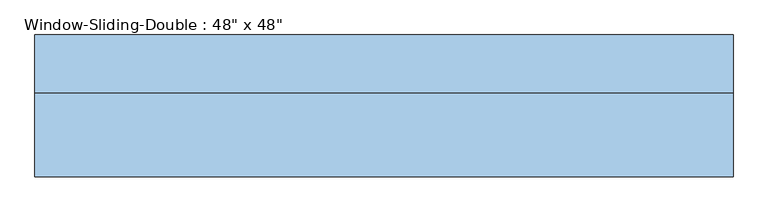
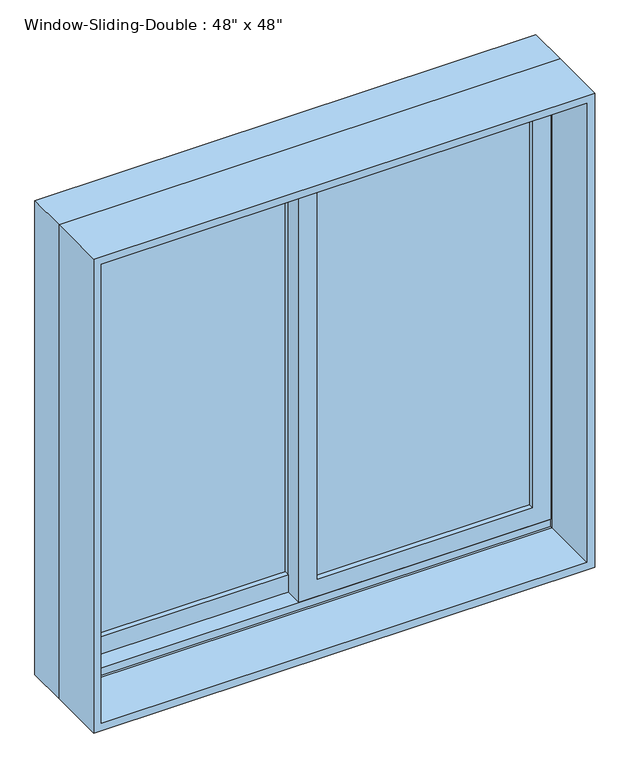
"""IFC4 building model written with IfcOpenShell, lengths in millimetres: window geometry."""

from ifc_helpers import new_model, si_unit, frame, origin, place, context, project, spatial, polyline, outline, extrude, faceted_brep, source, transform, mapped, element, save


def window_5af5dca6(model_context):
    return source(origin(), model_context, "Body", "SolidModel", [
        extrude(outline(polyline([(952.5, 590.55), (2114.55, 590.55), (2114.55, -22.225), (952.5, -22.225), (952.5, 590.55)]), holes=[polyline([(996.95, 22.225), (2070.1, 22.225), (2070.1, 546.1), (996.95, 546.1), (996.95, 22.225)])]), frame((0.0, 34.29, 0.0), z_axis=(0.0, 1.0, 0.0), x_axis=(0.0, 0.0, 1.0)), (0.0, 0.0, 1.0), 44.45),
        extrude(outline(polyline([(933.45, -590.55), (933.45, 22.225), (2114.55, 22.225), (2114.55, -590.55), (933.45, -590.55)]), holes=[polyline([(2070.1, -22.225), (996.95, -22.225), (996.95, -546.1), (2070.1, -546.1), (2070.1, -22.225)])]), frame((0.0, 78.74, 0.0), z_axis=(0.0, 1.0, 0.0), x_axis=(0.0, 0.0, 1.0)), (0.0, 0.0, 1.0), 44.45),
        extrude(outline(polyline([(-22.225, 110.49), (-22.225, 104.14), (-546.1, 104.14), (-546.1, 110.49), (-22.225, 110.49)])), frame((0.0, 0.0, 996.95), z_axis=(0.0, 0.0, 1.0), x_axis=(1.0, 0.0, 0.0)), (0.0, 0.0, 1.0), 1073.15),
        extrude(outline(polyline([(-22.225, 97.79), (-22.225, 91.44), (-546.1, 91.44), (-546.1, 97.79), (-22.225, 97.79)])), frame((0.0, 0.0, 996.95), z_axis=(0.0, 0.0, 1.0), x_axis=(1.0, 0.0, 0.0)), (0.0, 0.0, 1.0), 1073.15),
        extrude(outline(polyline([(546.1, 66.04), (546.1, 59.69), (22.225, 59.69), (22.225, 66.04), (546.1, 66.04)])), frame((0.0, 0.0, 996.95), z_axis=(0.0, 0.0, 1.0), x_axis=(1.0, 0.0, 0.0)), (0.0, 0.0, 1.0), 1073.15),
        extrude(outline(polyline([(546.1, 53.34), (546.1, 46.99), (22.225, 46.99), (22.225, 53.34), (546.1, 53.34)])), frame((0.0, 0.0, 996.95), z_axis=(0.0, 0.0, 1.0), x_axis=(1.0, 0.0, 0.0)), (0.0, 0.0, 1.0), 1073.15),
        extrude(outline(polyline([(2133.6, -609.6), (914.4, -609.6), (914.4, 609.6), (2133.6, 609.6), (2133.6, -609.6)]), holes=[polyline([(2114.55, 590.55), (933.45, 590.55), (933.45, -590.55), (2114.55, -590.55), (2114.55, 590.55)])]), frame((0.0, -118.11, 0.0), z_axis=(0.0, 1.0, 0.0), x_axis=(0.0, 0.0, 1.0)), (0.0, 0.0, 1.0), 146.05),
        faceted_brep([(-609.6, 27.94, 914.4), (-609.6, 129.54, 914.4), (609.6, 129.54, 914.4), (609.6, 27.94, 914.4), (-568.6778905, 129.54, 2092.6778905), (-568.6778905, 123.19, 2092.6778905), (-568.6778905, 123.19, 933.45), (-568.6778905, 129.54, 933.45), (568.6778905, 123.19, 2092.6778905), (568.6778905, 123.19, 933.45), (590.55, 123.19, 933.45), (590.55, 123.19, 2114.55), (-590.55, 123.19, 2114.55), (-590.55, 123.19, 933.45), (-590.55, 27.94, 2114.55), (-590.55, 27.94, 933.45), (-590.55, 34.29, 933.45), (-590.55, 34.29, 952.5), (-590.55, 78.74, 952.5), (-590.55, 78.74, 933.45), (609.6, 27.94, 2133.6), (-609.6, 27.94, 2133.6), (590.55, 27.94, 2114.55), (590.55, 27.94, 933.45), (-609.6, 129.54, 2133.6), (609.6, 129.54, 2133.6), (568.6778905, 129.54, 933.45), (568.6778905, 129.54, 2092.6778905), (590.55, 78.74, 933.45), (590.55, 78.74, 952.5), (590.55, 34.29, 952.5), (590.55, 34.29, 933.45)], [[[0, 1, 2, 3]], [[4, 5, 6, 7]], [[5, 8, 9, 10, 11, 12, 13, 6]], [[12, 14, 15, 16, 17, 18, 19, 13]], [[0, 3, 20, 21], [22, 23, 15, 14]], [[24, 1, 0, 21]], [[2, 1, 24, 25], [4, 7, 26, 27]], [[5, 4, 27, 8]], [[12, 11, 22, 14]], [[21, 20, 25, 24]], [[8, 27, 26, 9]], [[22, 11, 10, 28, 29, 30, 31, 23]], [[20, 3, 2, 25]], [[26, 7, 6, 13, 19, 28, 10, 9]], [[28, 19, 18, 29]], [[29, 18, 17, 30]], [[30, 17, 16, 31]], [[15, 23, 31, 16]]]),
    ])


if __name__ == "__main__":
    model = new_model("IFC4")
    model_context = context("Model", 3, world=origin())
    ifc_project = project(units=[si_unit("LENGTHUNIT", "METRE", prefix="MILLI")], contexts=[model_context])
    site = spatial("IfcSite", under=ifc_project)
    building = spatial("IfcBuilding", under=site)
    placement = place(None, origin())
    window_shape = window_5af5dca6(model_context)
    element("IfcWindow", 1, ObjectType="Window-Sliding-Double : 48\" x 48\"", at=placement, inside=building, context=model_context, shape_type="MappedRepresentation", body=[
        mapped(window_shape, transform((0.0, 0.0, 0.0), x_axis=(1.0, 0.0, 0.0), y_axis=(0.0, 1.0, 0.0), z_axis=(0.0, 0.0, 1.0))),
    ])
    save(model, "model.ifc")

# Revit data of these elements
# Type "Window-Sliding-Double : 48\" x 48\""
#   Type Mark = "23"
#   Fire Rating = "0.5h"
#   Assembly Code = "B2020100"
#   Analytic Construction = "Double glazing - domestic"
#   Window Inset [instance default] = 0' - 0"
#   Wall Thickness [instance default] = 0' - 6"
#   Visual Light Transmittance = 0.81
#   Thermal Resistance (R) = 1.8146 (h·ft²·°F)/BTU
#   Solar Heat Gain Coefficient = 0.76
#   Muntin Width = 1' - 8 5/8"
#   Muntin Height = 3' - 6 1/4"
#   Interior Wall Closure [instance default] = 0' - 2 3/4"
#   Heat Transfer Coefficient (U) = 0.5511 BTU/(h·ft²·°F)
#   Frame Extension [instance default] = 0' - 0 1/4"
#   Exterior Wall Closure [instance default] = 0' - 1 1/4"
#   Rough Width = 4' - 0 1/2"
#   Rough Height = 4' - 0 1/2"
#   Height = 4' - 0"
#   Extension Jamb [instance default] = 0' - 2 3/4"
#   Default Sill Height = 3' - 0"
#   Width = 4' - 0"
#   Interior Trim Visibility [instance default] = yes
#   Indicator Visibility [instance default] = yes
#   Exterior Trim Visibility [instance default] = yes
#   Muntin Visibility = yes
#   Extension Jamb Visibility [instance default] = yes
#   Muntin Pattern = Muntin Pattern_2x2 : Muntin Pattern_2x2
#   Interior Trim Material = Wood - Stained
#   Interior Trim = Trim-Window-Interior-Flat : Picture Frame
#   Interior Frame Material = Wood - Stained
#   Glass Panel Material = Glass
#   Exterior Trim Material = Clad - White
#   Exterior Trim = Trim-Window-Exterior-Flat : with Sill
#   Exterior Frame Material = Clad - White
#   Wall Closure = (empty or 0)
# Element 1 (IfcWindow, "Window-Sliding-Double : 48\" x 48\"")
#   Wall Thickness = 0' - 9"
#   Extension Jamb = 0' - 5 3/4"
#   Materials on its faces: "Wood - Stained", "Glass", "Clad - White"
# Materials
#   "Wood - Stained": class "Wood", colour RGB 224 178 126, transparency 0, Cost = 0
#   "Glass": class "Glass", colour RGB 0 128 192, transparency 0.75, Description = "Soda Lime Glass", Cost = 0
#   "Clad - White": class "Wood", colour RGB 242 242 238, transparency 0, Cost = 0
